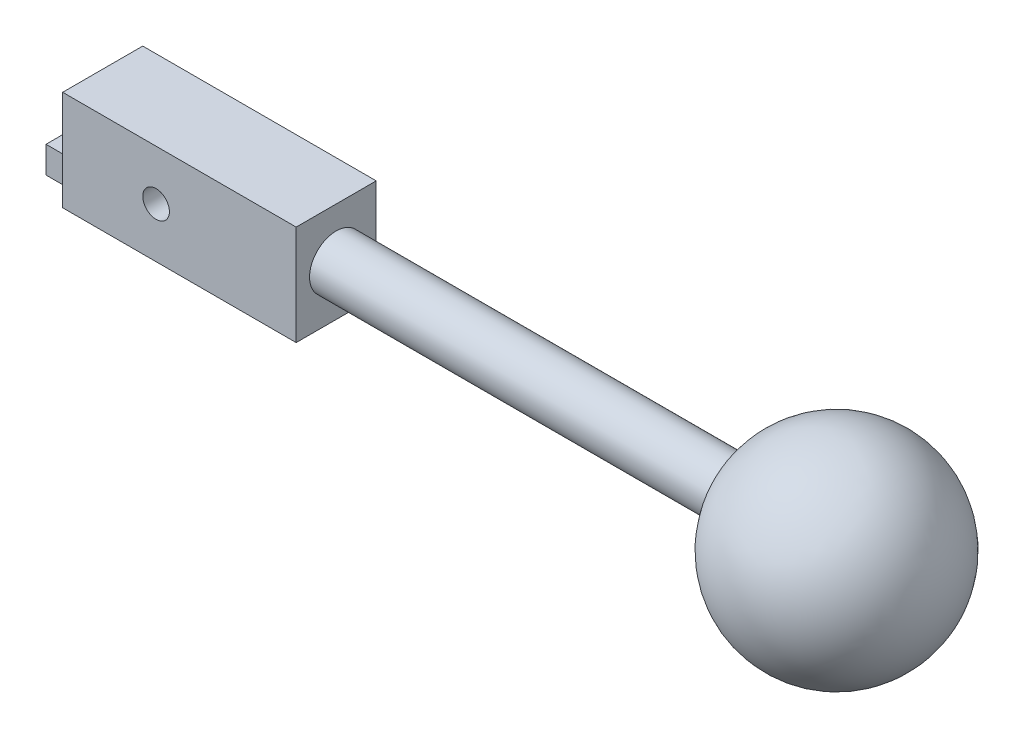
from build123d import *

# Parameters (mm, degrees)
HUB_BLOCK_SKETCH_W = 35
HUB_BLOCK_SKETCH_H = 15
HUB_BLOCK_DEPTH    = 12
DRIVE_TAB_SKETCH_W = 6
DRIVE_TAB_SKETCH_H = 4
DRIVE_TAB_DEPTH    = 5.5
SHAFT_SKETCH_R     = 4
SHAFT_8_DEPTH      = 75
PIN_HOLE_SKETCH_R  = 2
PIN_HOLE_4_DEPTH   = 75


with BuildPart() as part:
    # Hub Block Sketch → Hub Block (new body)
    with BuildSketch(Plane.XY):
        Rectangle(HUB_BLOCK_SKETCH_W, HUB_BLOCK_SKETCH_H)
    extrude(amount=HUB_BLOCK_DEPTH)

    # Drive Tab Sketch → Drive Tab (add)
    with BuildSketch(Plane.ZY.offset(17.5)):
        with Locations((6, -5.5)):
            Rectangle(DRIVE_TAB_SKETCH_W, DRIVE_TAB_SKETCH_H)
    extrude(amount=DRIVE_TAB_DEPTH)

    # Shaft Sketch → Shaft Ø8 (add)
    with BuildSketch(Plane(origin=(17.5, 0, 0), x_dir=(0, 0, -1), z_dir=(1, 0, 0))):
        with Locations((-6, 0)):
            Circle(SHAFT_SKETCH_R)
    extrude(amount=SHAFT_8_DEPTH)

    # Ball Knob Sketch → Ball Knob Ø30 (revolve)
    with BuildSketch(Plane(origin=(0, 0, 0), x_dir=(1, 0, 0), z_dir=(0, 1, 0))):
        with BuildLine():
            Line((92.5, 9), (92.5, -21))
            ThreePointArc((92.5, -21), (107.5, -6), (92.5, 9))
        make_face()
    revolve(axis=Axis((92.5, 0, 0), (0, 0, 1)))

    # Pin Hole Sketch → Pin Hole Ø4 (cut)
    with BuildSketch(Plane.XY.offset(12)):
        with Locations((-3.5, 0)):
            Circle(PIN_HOLE_SKETCH_R)
    extrude(amount=-PIN_HOLE_4_DEPTH, mode=Mode.SUBTRACT)


solid = part.part
